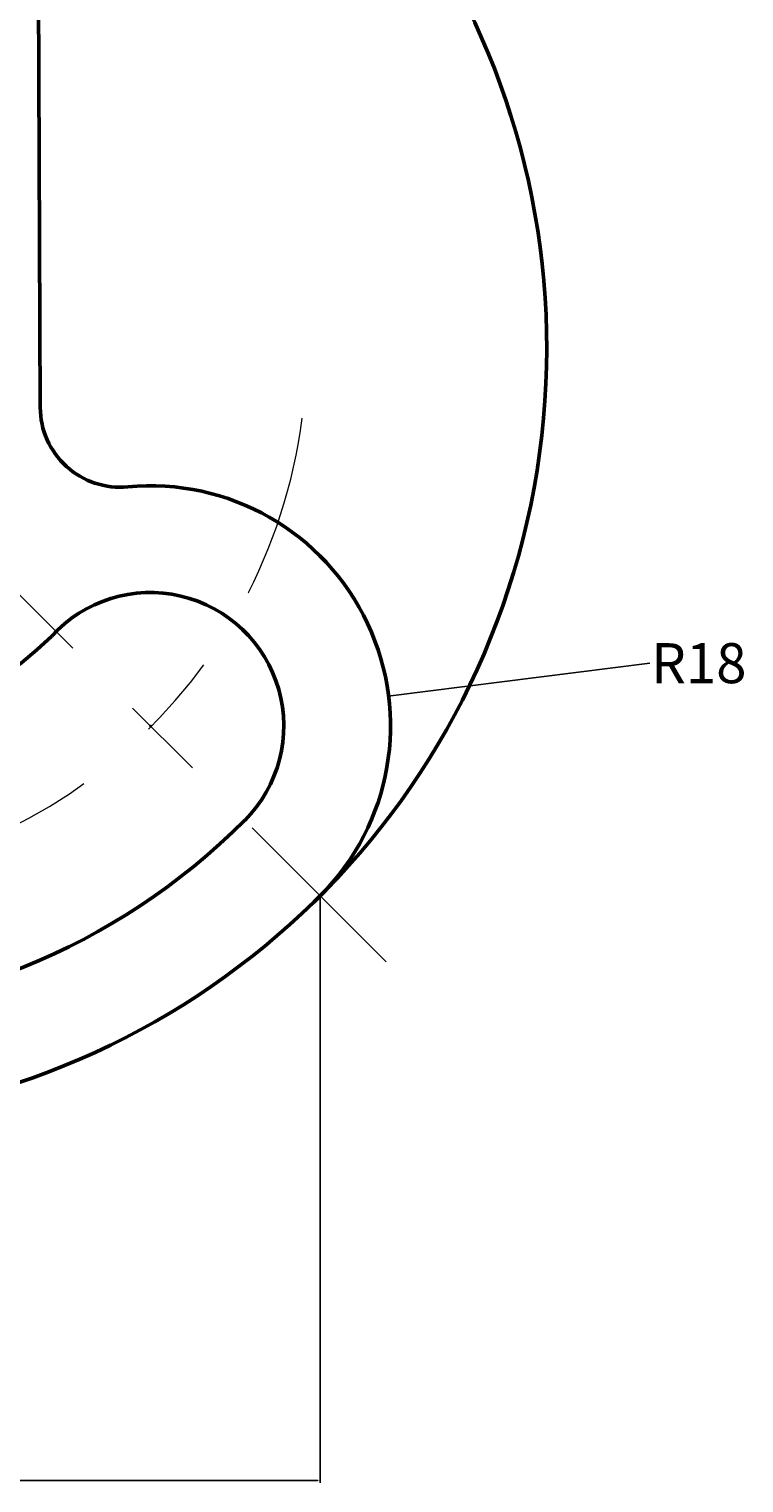
# Model space of a CAD drawing. Units: millimetres. Extents: x -53 to 92, y -147 to 37.
# Tile 9 of 16: x 38 to 92, y -139 to -30. Entities that reach past the tile are written whole.
import ezdxf

# ---------------------------------------------------------------- set-up
doc = ezdxf.new("R2010")
doc.units = ezdxf.units.MM
doc.header["$MEASUREMENT"] = 0
doc.linetypes.add('CENTER', pattern=[50.8, 31.75, -6.35, 6.35, -6.35])
for name, color, linetype, lineweight in [('M-CNTR', 4, 'CENTER', 18), ('M-DIMS', 2, 'Continuous', 25), ('M-OUTL', 7, 'Continuous', 50)]:
    doc.layers.add(name, color=color, linetype=linetype, lineweight=lineweight)
doc.styles.get("Standard").update_dxf_attribs({"font": 'arial.ttf'})
doc.dimstyles.get("Standard").update_dxf_attribs({"dimtxt": 0.18, "dimasz": 0.18, "dimexe": 0.18, "dimexo": 0.0625, "dimgap": 0.09, "dimtad": 0, "dimtih": 1, "dimtoh": 1, "dimdec": 4, "dimzin": 0, "dimdsep": 46, "dimtxsty": 'Standard', "dimcen": 0.09, "dimadec": 0, "dimazin": 0, "dimtfac": 1, "dimtdec": 4, "dimtofl": 0, "dimtmove": 0, "dimatfit": 3, "dimfxl": 1, "dimtolj": 1, "dimtzin": 0, "dimarcsym": 0})

# ---------------------------------------------------------------- blocks, each defined once
blk = doc.blocks.new('*D10')
at = {"layer": 'Defpoints', "color": 0, "transparency": 16777216}
for p in [(64.59, -18.18), (-26.68, -89.78)]:
    blk.add_point(p, dxfattribs=at)
at = {"layer": 'M-DIMS', "color": 0, "lineweight": -2, "transparency": 16777216}
for p, q in [((77.38, -8.15), (64.73, -18.07)), ((77.56, -8.15), (77.38, -8.15)), ((18.87, -53.98), (19.05, -53.98)), ((18.96, -54.07), (18.96, -53.89))]:
    blk.add_line(p, q, dxfattribs=at)
at = {"layer": 'M-DIMS', "color": 0, "transparency": 16777216}
blk.add_solid([(64.72, -18.05), (64.75, -18.1), (64.59, -18.18)], dxfattribs=at)
at = {"layer": 'M-DIMS', "color": 0, "transparency": 16777216, "insert": (82.6, -8.15), "char_height": 0.18, "attachment_point": 5}
blk.add_mtext('\\A1;{\\H16.66667x;%%C116}', dxfattribs=at)
blk = doc.blocks.new('*D11')
at = {"layer": 'Defpoints', "color": 0, "transparency": 16777216}
for p in [(65.1, -80.02), (47.24, -82.26)]:
    blk.add_point(p, dxfattribs=at)
at = {"layer": 'M-DIMS', "color": 0, "lineweight": -2, "transparency": 16777216}
for p, q in [((84.69, -77.56), (65.28, -80)), ((47.15, -82.26), (47.33, -82.26)), ((47.24, -82.35), (47.24, -82.17))]:
    blk.add_line(p, q, dxfattribs=at)
at = {"layer": 'M-DIMS', "color": 0, "transparency": 16777216}
blk.add_solid([(65.28, -79.97), (65.28, -80.03), (65.1, -80.02)], dxfattribs=at)
at = {"layer": 'M-DIMS', "color": 0, "transparency": 16777216, "insert": (88.37, -77.56), "char_height": 0.18, "attachment_point": 5}
blk.add_mtext('\\A1;{\\H16.66667x;R18}', dxfattribs=at)
blk = doc.blocks.new('*D16')
at = {"layer": 'Defpoints', "color": 0, "transparency": 16777216}
for p in [(-22.06, -94.99), (59.97, -94.99), (59.97, -138.81)]:
    blk.add_point(p, dxfattribs=at)
at = {"layer": 'M-DIMS', "color": 0, "lineweight": -2, "transparency": 16777216}
for p, q in [((-22.06, -95.05), (-22.06, -138.99)), ((59.97, -95.05), (59.97, -138.99)), ((-21.88, -138.81), (18.56, -138.81)), ((59.79, -138.81), (19.35, -138.81))]:
    blk.add_line(p, q, dxfattribs=at)
at = {"layer": 'M-DIMS', "color": 0, "transparency": 16777216}
for points in [[(-21.88, -138.78), (-21.88, -138.84), (-22.06, -138.81)], [(59.79, -138.78), (59.79, -138.84), (59.97, -138.81)]]:
    blk.add_solid(points, dxfattribs=at)
at = {"layer": 'M-DIMS', "color": 0, "transparency": 16777216, "insert": (18.96, -138.81), "char_height": 0.18, "attachment_point": 5}
blk.add_mtext('\\A1;82.02', dxfattribs=at)

msp = doc.modelspace()

# ---------------------------------------------------------------- linework, layer by layer
at = {"layer": 'M-CNTR'}
msp.add_line((18.95638, -53.98007), (64.91832, -99.94201), dxfattribs=at)
msp.add_arc((18.95638, -54.07007), 40, 187.3659151, 352.6278316, dxfattribs=at)
at = {"layer": 'M-OUTL'}
msp.add_line((38.69188, 15.90293), (38.97226, -58.39443), dxfattribs=at)
for centre, radius, start, end in [((18.95638, -53.98007), 58, 108.3895553, 70.0459142), ((44.97222, -58.37178), 6, 180.2162159, 275.4235757), ((47.24065, -82.26434), 18, 315.0000023, 95.4235757), ((47.24065, -82.26434), 10, 314.9623781, 137.789666), ((18.95638, -53.98007), 30.01579, 315.9289422, 315.9290723), ((18.95638, -53.98007), 30.01579, 225.9289422, 314.0710578), ((18.95621, -53.96903), 50.00792, 225.0090785, 314.9943099)]:
    msp.add_arc(centre, radius, start, end, dxfattribs=at)

# ---------------------------------------------------------------- dimensions: what is measured, and where the dimension line sits
at = {"layer": 'M-DIMS'}
dim = msp.add_diameter_dim_2p(p1=(-26.67986, -89.77579), p2=(64.59262, -18.18435), text='{\\H16.66667x;%%C116}', dimstyle='Standard', override={"dimclrd": 0, "dimclre": 0, "dimclrt": 0}, dxfattribs=at)
dim.commit()
dim.dimension.update_dxf_attribs({"geometry": '*D10', "text_midpoint": (82.59889, -8.15132), "dimtype": 163})
dim = msp.add_radius_dim(center=(47.24065, -82.26434), mpoint=(65.10018, -80.01999), text='{\\H16.66667x;R18}', dimstyle='Standard', override={"dimclrd": 0, "dimclre": 0, "dimclrt": 0}, dxfattribs=at)
dim.commit()
dim.dimension.update_dxf_attribs({"geometry": '*D11', "text_midpoint": (84.69084, -77.55809), "dimtype": 164})
dim = msp.add_linear_dim(base=(59.96857, -138.81235), p1=(-22.0558, -94.99225), p2=(59.96857, -94.99226), dimstyle='Standard', override={"dimdec": 2, "dimlfac": 1, "dimrnd": 0, "dimzin": 0, "dimdsep": 46, "dimlunit": 2}, dxfattribs=at)
dim.commit()
dim.dimension.update_dxf_attribs({"geometry": '*D16', "text_midpoint": (18.95639, -138.81235)})

doc.saveas('drawing.dxf')
